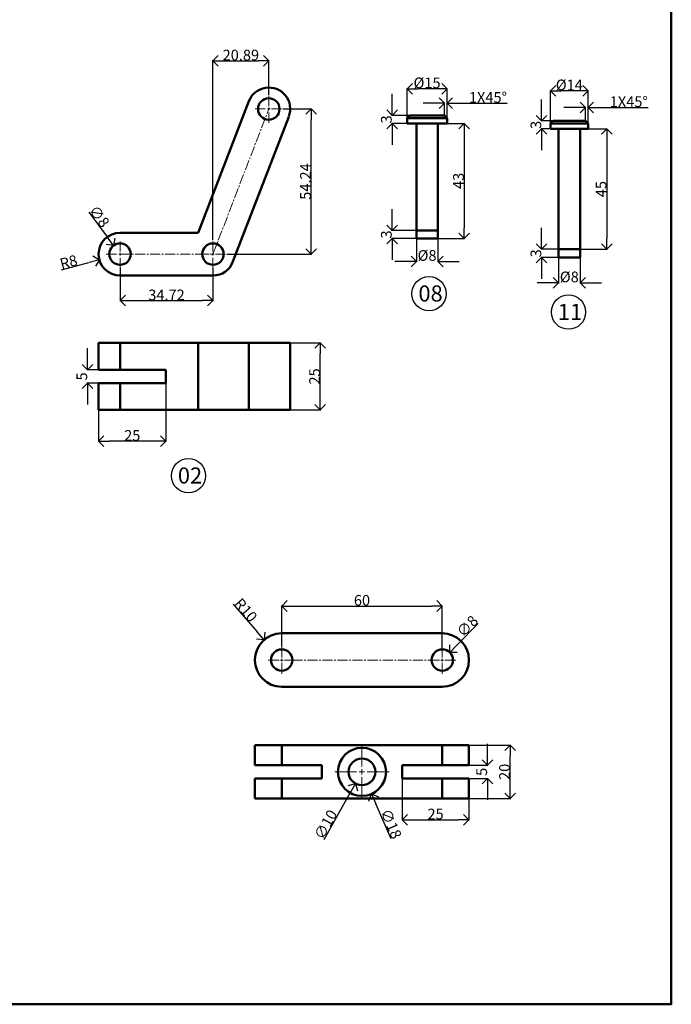
# Model space of a CAD drawing. Units: millimetres. Extents: x 45 to 546, y 51 to 638.
# Tile 2 of 4: x 303 to 546, y 51 to 419. Entities that reach past the tile are written whole.
import ezdxf

# ---------------------------------------------------------------- set-up
doc = ezdxf.new("R2010")
doc.units = ezdxf.units.MM
doc.header["$MEASUREMENT"] = 0
doc.linetypes.add('CENTER2', pattern=[1.125, 0.75, -0.125, 0.125, -0.125])
for name, color, linetype, lineweight in [('M-CNTR', 1, 'CENTER2', 18), ('M-DIMS', 2, 'Continuous', 25), ('M-OUTL', 7, 'Continuous', 50), ('M-TEXT', 7, 'Continuous', 25), ('M-TTLB', 7, 'Continuous', 50)]:
    doc.layers.add(name, color=color, linetype=linetype, lineweight=lineweight)
doc.styles.get("Standard").update_dxf_attribs({"font": 'arial.ttf'})
doc.dimstyles.get("Standard").update_dxf_attribs({"dimtxt": 4, "dimasz": 4, "dimexe": 0.18, "dimexo": 0.0625, "dimgap": 0.09, "dimtad": 1, "dimdec": 0, "dimzin": 0, "dimdsep": 46, "dimtxsty": 'Standard', "dimblk": 'OPEN90', "dimcen": 0.09, "dimclre": 251, "dimadec": 0, "dimazin": 0, "dimtfac": 1, "dimtdec": 0, "dimtofl": 0, "dimtmove": 0, "dimatfit": 3, "dimfxl": 1, "dimtolj": 1, "dimtzin": 0, "dimarcsym": 0})

# ---------------------------------------------------------------- blocks, each defined once
blk = doc.blocks.new('_Open90')
at = {"color": 0, "linetype": 'ByBlock', "lineweight": -2}
for p, q in [((0, 0), (-1, 0)), ((-0.5, 0.5), (0, 0)), ((0, 0), (-0.5, -0.5))]:
    blk.add_line(p, q, dxfattribs=at)
blk = doc.blocks.new('*D54')
at = {"layer": 'Defpoints', "color": 0, "transparency": 16777216}
for p in [(337.79, 334.56), (342.59, 328.16)]:
    blk.add_point(p, dxfattribs=at)
at = {"layer": 'M-DIMS', "color": 0, "lineweight": -2, "transparency": 16777216}
for p, q in [((328.48, 346.98), (335.39, 337.76)), ((340.1, 331.36), (340.28, 331.36)), ((340.19, 331.27), (340.19, 331.45))]:
    blk.add_line(p, q, dxfattribs=at)
at = {"layer": 'M-DIMS', "color": 0, "lineweight": -2, "transparency": 16777216, "xscale": 4, "yscale": 4, "zscale": 4, "rotation": 306.8480275512002}
blk.add_blockref('_Open90', (337.79, 334.56), dxfattribs=at)
at = {"layer": 'M-DIMS', "color": 0, "transparency": 16777216, "insert": (332.42, 345.46), "char_height": 4, "attachment_point": 5, "rotation": 306.848}
blk.add_mtext('\\A1;∅8', dxfattribs=at)
blk = doc.blocks.new('*D55')
at = {"layer": 'Defpoints', "color": 0, "transparency": 16777216}
for p in [(340.19, 331.36), (332.46, 329.29)]:
    blk.add_point(p, dxfattribs=at)
at = {"layer": 'M-DIMS', "color": 0, "lineweight": -2, "transparency": 16777216}
for p, q in [((340.1, 331.36), (340.28, 331.36)), ((340.19, 331.27), (340.19, 331.45)), ((318.32, 325.51), (328.59, 328.26))]:
    blk.add_line(p, q, dxfattribs=at)
at = {"layer": 'M-DIMS', "color": 0, "lineweight": -2, "transparency": 16777216, "xscale": 4, "yscale": 4, "zscale": 4, "rotation": 14.96151981940441}
blk.add_blockref('_Open90', (332.46, 329.29), dxfattribs=at)
at = {"layer": 'M-DIMS', "color": 0, "transparency": 16777216, "insert": (320.97, 328.43), "char_height": 4, "attachment_point": 5, "rotation": 14.9615}
blk.add_mtext('\\A1;R8', dxfattribs=at)
blk = doc.blocks.new('*U56')
at = {"layer": 'M-CNTR', "color": 0, "ltscale": 5, "transparency": 16777216}
for p, q in [((0, 1), (0, 5.12)), ((-5.12, 0), (-1, 0)), ((1, 0), (5.12, 0)), ((0, -5.12), (0, -1))]:
    blk.add_line(p, q, dxfattribs=at)
at = {"layer": 'M-CNTR', "color": 0, "linetype": 'Continuous', "ltscale": 5, "transparency": 16777216}
for p, q in [((-0.5, 0), (0.5, 0)), ((0, -0.5), (0, 0.5))]:
    blk.add_line(p, q, dxfattribs=at)
blk = doc.blocks.new('*U57')
at = {"layer": 'M-CNTR', "color": 0, "ltscale": 5, "transparency": 16777216}
for p, q in [((0, 1), (0, 5.12)), ((-5.12, 0), (-1, 0)), ((1, 0), (5.12, 0)), ((0, -5.12), (0, -1))]:
    blk.add_line(p, q, dxfattribs=at)
at = {"layer": 'M-CNTR', "color": 0, "linetype": 'Continuous', "ltscale": 5, "transparency": 16777216}
for p, q in [((-0.5, 0), (0.5, 0)), ((0, -0.5), (0, 0.5))]:
    blk.add_line(p, q, dxfattribs=at)
blk = doc.blocks.new('*U58')
at = {"layer": 'M-CNTR', "color": 0, "ltscale": 5, "transparency": 16777216}
for p, q in [((0, 1), (0, 5.12)), ((-5.12, 0), (-1, 0)), ((1, 0), (5.12, 0)), ((0, -5.12), (0, -1))]:
    blk.add_line(p, q, dxfattribs=at)
at = {"layer": 'M-CNTR', "color": 0, "linetype": 'Continuous', "ltscale": 5, "transparency": 16777216}
for p, q in [((-0.5, 0), (0.5, 0)), ((0, -0.5), (0, 0.5))]:
    blk.add_line(p, q, dxfattribs=at)
blk = doc.blocks.new('*D59')
at = {"layer": 'Defpoints', "color": 0, "transparency": 16777216}
for p in [(340.19, 326.24), (374.91, 326.24), (374.91, 313.98)]:
    blk.add_point(p, dxfattribs=at)
at = {"layer": 'M-DIMS', "color": 0, "lineweight": -2, "transparency": 16777216}
for p, q in [((340.19, 326.18), (340.19, 313.8)), ((374.91, 326.18), (374.91, 313.8)), ((344.19, 313.98), (370.91, 313.98))]:
    blk.add_line(p, q, dxfattribs=at)
at = {"layer": 'M-DIMS', "color": 0, "lineweight": -2, "transparency": 16777216, "xscale": 4, "yscale": 4, "zscale": 4, "rotation": 180}
blk.add_blockref('_Open90', (340.19, 313.98), dxfattribs=at)
at = {"layer": 'M-DIMS', "color": 0, "lineweight": -2, "transparency": 16777216, "xscale": 4, "yscale": 4, "zscale": 4}
blk.add_blockref('_Open90', (374.91, 313.98), dxfattribs=at)
at = {"layer": 'M-DIMS', "color": 0, "transparency": 16777216, "insert": (357.55, 316.11), "char_height": 4, "attachment_point": 5}
blk.add_mtext('\\A1;34.72', dxfattribs=at)
blk = doc.blocks.new('*D60')
at = {"layer": 'Defpoints', "color": 0, "transparency": 16777216}
for p in [(400.92, 385.6), (411.64, 385.6), (380.03, 331.36)]:
    blk.add_point(p, dxfattribs=at)
at = {"layer": 'M-DIMS', "color": 0, "lineweight": -2, "transparency": 16777216}
for p, q in [((400.98, 385.6), (411.82, 385.6)), ((411.64, 335.36), (411.64, 381.6)), ((380.09, 331.36), (411.82, 331.36))]:
    blk.add_line(p, q, dxfattribs=at)
at = {"layer": 'M-DIMS', "color": 0, "lineweight": -2, "transparency": 16777216, "xscale": 4, "yscale": 4, "zscale": 4}
for p, rotation in [((411.64, 385.6), 90), ((411.64, 331.36), 270)]:
    blk.add_blockref('_Open90', p, dxfattribs=dict(at, rotation=rotation))
at = {"layer": 'M-DIMS', "color": 0, "transparency": 16777216, "insert": (409.5, 358.48), "char_height": 4, "attachment_point": 5, "rotation": 90}
blk.add_mtext('\\A1;54.24', dxfattribs=at)
blk = doc.blocks.new('*D61')
at = {"layer": 'Defpoints', "color": 0, "transparency": 16777216}
for p in [(395.8, 403.6), (395.8, 390.72), (374.91, 336.48)]:
    blk.add_point(p, dxfattribs=at)
at = {"layer": 'M-DIMS', "color": 0, "lineweight": -2, "transparency": 16777216}
for p, q in [((374.91, 336.54), (374.91, 403.78)), ((378.91, 403.6), (391.8, 403.6)), ((395.8, 390.78), (395.8, 403.78))]:
    blk.add_line(p, q, dxfattribs=at)
at = {"layer": 'M-DIMS', "color": 0, "lineweight": -2, "transparency": 16777216, "xscale": 4, "yscale": 4, "zscale": 4, "rotation": 180}
blk.add_blockref('_Open90', (374.91, 403.6), dxfattribs=at)
at = {"layer": 'M-DIMS', "color": 0, "lineweight": -2, "transparency": 16777216, "xscale": 4, "yscale": 4, "zscale": 4}
blk.add_blockref('_Open90', (395.8, 403.6), dxfattribs=at)
at = {"layer": 'M-DIMS', "color": 0, "transparency": 16777216, "insert": (385.35, 405.73), "char_height": 4, "attachment_point": 5}
blk.add_mtext('\\A1;20.89', dxfattribs=at)
blk = doc.blocks.new('*D62')
at = {"layer": 'Defpoints', "color": 0, "transparency": 16777216}
for p in [(328.02, 288.16), (332.19, 288.16), (332.19, 283.16)]:
    blk.add_point(p, dxfattribs=at)
at = {"layer": 'M-DIMS', "color": 0, "lineweight": -2, "transparency": 16777216}
for p, q in [((328.02, 292.16), (328.02, 296.16)), ((332.13, 288.16), (327.84, 288.16)), ((332.13, 283.16), (327.84, 283.16)), ((328.02, 279.16), (328.02, 275.16))]:
    blk.add_line(p, q, dxfattribs=at)
at = {"layer": 'M-DIMS', "color": 0, "lineweight": -2, "transparency": 16777216, "xscale": 4, "yscale": 4, "zscale": 4}
for p, rotation in [((328.02, 288.16), 270), ((328.02, 283.16), 90)]:
    blk.add_blockref('_Open90', p, dxfattribs=dict(at, rotation=rotation))
at = {"layer": 'M-DIMS', "color": 0, "transparency": 16777216, "insert": (325.9, 285.66), "char_height": 4, "attachment_point": 5, "rotation": 90}
blk.add_mtext('\\A1;5', dxfattribs=at)
blk = doc.blocks.new('*D63')
at = {"layer": 'Defpoints', "color": 0, "transparency": 16777216}
for p in [(357.34, 283.16), (332.19, 273.16), (332.19, 261.47)]:
    blk.add_point(p, dxfattribs=at)
at = {"layer": 'M-DIMS', "color": 0, "lineweight": -2, "transparency": 16777216}
for p, q in [((357.34, 283.1), (357.34, 261.29)), ((332.19, 273.1), (332.19, 261.29)), ((353.34, 261.47), (336.19, 261.47))]:
    blk.add_line(p, q, dxfattribs=at)
at = {"layer": 'M-DIMS', "color": 0, "lineweight": -2, "transparency": 16777216, "xscale": 4, "yscale": 4, "zscale": 4, "rotation": 180}
blk.add_blockref('_Open90', (332.19, 261.47), dxfattribs=at)
at = {"layer": 'M-DIMS', "color": 0, "lineweight": -2, "transparency": 16777216, "xscale": 4, "yscale": 4, "zscale": 4}
blk.add_blockref('_Open90', (357.34, 261.47), dxfattribs=at)
at = {"layer": 'M-DIMS', "color": 0, "transparency": 16777216, "insert": (344.76, 263.6), "char_height": 4, "attachment_point": 5}
blk.add_mtext('\\A1;25', dxfattribs=at)
blk = doc.blocks.new('*D64')
at = {"layer": 'Defpoints', "color": 0, "transparency": 16777216}
for p in [(403.8, 298.16), (415.04, 298.16), (403.8, 273.16)]:
    blk.add_point(p, dxfattribs=at)
at = {"layer": 'M-DIMS', "color": 0, "lineweight": -2, "transparency": 16777216}
for p, q in [((403.86, 298.16), (415.22, 298.16)), ((415.04, 277.16), (415.04, 294.16)), ((403.86, 273.16), (415.22, 273.16))]:
    blk.add_line(p, q, dxfattribs=at)
at = {"layer": 'M-DIMS', "color": 0, "lineweight": -2, "transparency": 16777216, "xscale": 4, "yscale": 4, "zscale": 4}
for p, rotation in [((415.04, 298.16), 90), ((415.04, 273.16), 270)]:
    blk.add_blockref('_Open90', p, dxfattribs=dict(at, rotation=rotation))
at = {"layer": 'M-DIMS', "color": 0, "transparency": 16777216, "insert": (412.91, 285.66), "char_height": 4, "attachment_point": 5, "rotation": 90}
blk.add_mtext('\\A1;25', dxfattribs=at)
blk = doc.blocks.new('*D65')
at = {"layer": 'Defpoints', "color": 0, "transparency": 16777216}
for p in [(441.87, 383.22), (448.45, 383.22), (447.45, 380.22)]:
    blk.add_point(p, dxfattribs=at)
at = {"layer": 'M-DIMS', "color": 0, "lineweight": -2, "transparency": 16777216}
for p, q in [((441.87, 387.22), (441.87, 391.22)), ((448.39, 383.22), (441.69, 383.22)), ((447.39, 380.22), (441.69, 380.22)), ((441.87, 376.22), (441.87, 372.22))]:
    blk.add_line(p, q, dxfattribs=at)
at = {"layer": 'M-DIMS', "color": 0, "lineweight": -2, "transparency": 16777216, "xscale": 4, "yscale": 4, "zscale": 4}
for p, rotation in [((441.87, 383.22), 270), ((441.87, 380.22), 90)]:
    blk.add_blockref('_Open90', p, dxfattribs=dict(at, rotation=rotation))
at = {"layer": 'M-DIMS', "color": 0, "transparency": 16777216, "insert": (439.73, 381.72), "char_height": 4, "attachment_point": 5, "rotation": 90}
blk.add_mtext('\\A1;3', dxfattribs=at)
blk = doc.blocks.new('*D66')
at = {"layer": 'Defpoints', "color": 0, "transparency": 16777216}
for p in [(441.87, 340.22), (450.95, 340.22), (450.95, 337.22)]:
    blk.add_point(p, dxfattribs=at)
at = {"layer": 'M-DIMS', "color": 0, "lineweight": -2, "transparency": 16777216}
for p, q in [((441.87, 344.22), (441.87, 348.22)), ((450.89, 340.22), (441.69, 340.22)), ((450.89, 337.22), (441.69, 337.22)), ((441.87, 333.22), (441.87, 329.22))]:
    blk.add_line(p, q, dxfattribs=at)
at = {"layer": 'M-DIMS', "color": 0, "lineweight": -2, "transparency": 16777216, "xscale": 4, "yscale": 4, "zscale": 4}
for p, rotation in [((441.87, 340.22), 270), ((441.87, 337.22), 90)]:
    blk.add_blockref('_Open90', p, dxfattribs=dict(at, rotation=rotation))
at = {"layer": 'M-DIMS', "color": 0, "transparency": 16777216, "insert": (439.73, 338.72), "char_height": 4, "attachment_point": 5, "rotation": 90}
blk.add_mtext('\\A1;3', dxfattribs=at)
blk = doc.blocks.new('*D67')
at = {"layer": 'Defpoints', "color": 0, "transparency": 16777216}
for p in [(462.45, 380.22), (458.95, 337.22), (468.81, 337.22)]:
    blk.add_point(p, dxfattribs=at)
at = {"layer": 'M-DIMS', "color": 0, "lineweight": -2, "transparency": 16777216}
for p, q in [((462.52, 380.22), (468.99, 380.22)), ((468.81, 376.22), (468.81, 341.22)), ((459.02, 337.22), (468.99, 337.22))]:
    blk.add_line(p, q, dxfattribs=at)
at = {"layer": 'M-DIMS', "color": 0, "lineweight": -2, "transparency": 16777216, "xscale": 4, "yscale": 4, "zscale": 4}
for p, rotation in [((468.81, 380.22), 90), ((468.81, 337.22), 270)]:
    blk.add_blockref('_Open90', p, dxfattribs=dict(at, rotation=rotation))
at = {"layer": 'M-DIMS', "color": 0, "transparency": 16777216, "insert": (466.68, 358.72), "char_height": 4, "attachment_point": 5, "rotation": 90}
blk.add_mtext('\\A1;43', dxfattribs=at)
blk = doc.blocks.new('*D68')
at = {"layer": 'Defpoints', "color": 0, "transparency": 16777216}
for p in [(450.95, 337.22), (458.95, 337.22), (450.95, 328.62)]:
    blk.add_point(p, dxfattribs=at)
at = {"layer": 'M-DIMS', "color": 0, "lineweight": -2, "transparency": 16777216}
for p, q in [((450.95, 337.16), (450.95, 328.44)), ((458.95, 337.16), (458.95, 328.44)), ((446.95, 328.62), (442.95, 328.62)), ((462.95, 328.62), (466.95, 328.62))]:
    blk.add_line(p, q, dxfattribs=at)
at = {"layer": 'M-DIMS', "color": 0, "lineweight": -2, "transparency": 16777216, "xscale": 4, "yscale": 4, "zscale": 4}
blk.add_blockref('_Open90', (450.95, 328.62), dxfattribs=at)
at = {"layer": 'M-DIMS', "color": 0, "lineweight": -2, "transparency": 16777216, "xscale": 4, "yscale": 4, "zscale": 4, "rotation": 180}
blk.add_blockref('_Open90', (458.95, 328.62), dxfattribs=at)
at = {"layer": 'M-DIMS', "color": 0, "transparency": 16777216, "insert": (454.95, 330.86), "char_height": 4, "attachment_point": 5}
blk.add_mtext('\\A1;%%C8', dxfattribs=at)
blk = doc.blocks.new('*D69')
at = {"layer": 'Defpoints', "color": 0, "transparency": 16777216}
for p in [(447.45, 393.11), (447.45, 382.22), (462.45, 382.22)]:
    blk.add_point(p, dxfattribs=at)
at = {"layer": 'M-DIMS', "color": 0, "lineweight": -2, "transparency": 16777216}
for p, q in [((447.45, 382.28), (447.45, 393.29)), ((458.45, 393.11), (451.45, 393.11)), ((462.45, 382.28), (462.45, 393.29))]:
    blk.add_line(p, q, dxfattribs=at)
at = {"layer": 'M-DIMS', "color": 0, "lineweight": -2, "transparency": 16777216, "xscale": 4, "yscale": 4, "zscale": 4, "rotation": 180}
blk.add_blockref('_Open90', (447.45, 393.11), dxfattribs=at)
at = {"layer": 'M-DIMS', "color": 0, "lineweight": -2, "transparency": 16777216, "xscale": 4, "yscale": 4, "zscale": 4}
blk.add_blockref('_Open90', (462.45, 393.11), dxfattribs=at)
at = {"layer": 'M-DIMS', "color": 0, "transparency": 16777216, "insert": (454.95, 395.35), "char_height": 4, "attachment_point": 5}
blk.add_mtext('\\A1;%%C15', dxfattribs=at)
blk = doc.blocks.new('*D70')
at = {"layer": 'Defpoints', "color": 0, "transparency": 16777216}
for p in [(462.45, 387.79), (461.45, 383.22), (462.45, 382.22)]:
    blk.add_point(p, dxfattribs=at)
at = {"layer": 'M-DIMS', "color": 0, "lineweight": -2, "transparency": 16777216}
for p, q in [((457.45, 387.79), (453.45, 387.79)), ((461.45, 383.28), (461.45, 387.97)), ((462.45, 382.28), (462.45, 387.97)), ((466.45, 387.79), (484.94, 387.79))]:
    blk.add_line(p, q, dxfattribs=at)
at = {"layer": 'M-DIMS', "color": 0, "lineweight": -2, "transparency": 16777216, "xscale": 4, "yscale": 4, "zscale": 4}
blk.add_blockref('_Open90', (461.45, 387.79), dxfattribs=at)
at = {"layer": 'M-DIMS', "color": 0, "lineweight": -2, "transparency": 16777216, "xscale": 4, "yscale": 4, "zscale": 4, "rotation": 180}
blk.add_blockref('_Open90', (462.45, 387.79), dxfattribs=at)
at = {"layer": 'M-DIMS', "color": 0, "transparency": 16777216, "insert": (477.7, 389.92), "char_height": 4, "attachment_point": 5}
blk.add_mtext('\\A1;1X45%%D', dxfattribs=at)
blk = doc.blocks.new('*D71')
at = {"layer": 'Defpoints', "color": 0, "transparency": 16777216}
for p in [(497.77, 333.16), (504.11, 333.16), (504.11, 330.16)]:
    blk.add_point(p, dxfattribs=at)
at = {"layer": 'M-DIMS', "color": 0, "lineweight": -2, "transparency": 16777216}
for p, q in [((497.77, 337.16), (497.77, 341.16)), ((504.05, 333.16), (497.59, 333.16)), ((504.05, 330.16), (497.59, 330.16)), ((497.77, 326.16), (497.77, 322.16))]:
    blk.add_line(p, q, dxfattribs=at)
at = {"layer": 'M-DIMS', "color": 0, "lineweight": -2, "transparency": 16777216, "xscale": 4, "yscale": 4, "zscale": 4}
for p, rotation in [((497.77, 333.16), 270), ((497.77, 330.16), 90)]:
    blk.add_blockref('_Open90', p, dxfattribs=dict(at, rotation=rotation))
at = {"layer": 'M-DIMS', "color": 0, "transparency": 16777216, "insert": (495.63, 331.66), "char_height": 4, "attachment_point": 5, "rotation": 90}
blk.add_mtext('\\A1;3', dxfattribs=at)
blk = doc.blocks.new('*D72')
at = {"layer": 'Defpoints', "color": 0, "transparency": 16777216}
for p in [(497.77, 381.16), (502.11, 381.16), (501.11, 378.16)]:
    blk.add_point(p, dxfattribs=at)
at = {"layer": 'M-DIMS', "color": 0, "lineweight": -2, "transparency": 16777216}
for p, q in [((497.77, 385.16), (497.77, 389.16)), ((502.05, 381.16), (497.59, 381.16)), ((501.05, 378.16), (497.59, 378.16)), ((497.77, 374.16), (497.77, 370.16))]:
    blk.add_line(p, q, dxfattribs=at)
at = {"layer": 'M-DIMS', "color": 0, "lineweight": -2, "transparency": 16777216, "xscale": 4, "yscale": 4, "zscale": 4}
for p, rotation in [((497.77, 381.16), 270), ((497.77, 378.16), 90)]:
    blk.add_blockref('_Open90', p, dxfattribs=dict(at, rotation=rotation))
at = {"layer": 'M-DIMS', "color": 0, "transparency": 16777216, "insert": (495.63, 379.66), "char_height": 4, "attachment_point": 5, "rotation": 90}
blk.add_mtext('\\A1;3', dxfattribs=at)
blk = doc.blocks.new('*D73')
at = {"layer": 'Defpoints', "color": 0, "transparency": 16777216}
for p in [(501.11, 392.34), (501.11, 380.16), (515.11, 380.16)]:
    blk.add_point(p, dxfattribs=at)
at = {"layer": 'M-DIMS', "color": 0, "lineweight": -2, "transparency": 16777216}
for p, q in [((501.11, 380.22), (501.11, 392.52)), ((511.11, 392.34), (505.11, 392.34)), ((515.11, 380.22), (515.11, 392.52))]:
    blk.add_line(p, q, dxfattribs=at)
at = {"layer": 'M-DIMS', "color": 0, "lineweight": -2, "transparency": 16777216, "xscale": 4, "yscale": 4, "zscale": 4, "rotation": 180}
blk.add_blockref('_Open90', (501.11, 392.34), dxfattribs=at)
at = {"layer": 'M-DIMS', "color": 0, "lineweight": -2, "transparency": 16777216, "xscale": 4, "yscale": 4, "zscale": 4}
blk.add_blockref('_Open90', (515.11, 392.34), dxfattribs=at)
at = {"layer": 'M-DIMS', "color": 0, "transparency": 16777216, "insert": (508.11, 394.58), "char_height": 4, "attachment_point": 5}
blk.add_mtext('\\A1;%%C14', dxfattribs=at)
blk = doc.blocks.new('*D74')
at = {"layer": 'Defpoints', "color": 0, "transparency": 16777216}
for p in [(515.11, 386.18), (514.11, 381.16), (515.11, 380.16)]:
    blk.add_point(p, dxfattribs=at)
at = {"layer": 'M-DIMS', "color": 0, "lineweight": -2, "transparency": 16777216}
for p, q in [((514.11, 381.22), (514.11, 386.36)), ((515.11, 380.22), (515.11, 386.36)), ((510.11, 386.18), (506.11, 386.18)), ((519.11, 386.18), (537.6, 386.18))]:
    blk.add_line(p, q, dxfattribs=at)
at = {"layer": 'M-DIMS', "color": 0, "lineweight": -2, "transparency": 16777216, "xscale": 4, "yscale": 4, "zscale": 4}
blk.add_blockref('_Open90', (514.11, 386.18), dxfattribs=at)
at = {"layer": 'M-DIMS', "color": 0, "lineweight": -2, "transparency": 16777216, "xscale": 4, "yscale": 4, "zscale": 4, "rotation": 180}
blk.add_blockref('_Open90', (515.11, 386.18), dxfattribs=at)
at = {"layer": 'M-DIMS', "color": 0, "transparency": 16777216, "insert": (530.35, 388.31), "char_height": 4, "attachment_point": 5}
blk.add_mtext('\\A1;1X45%%D', dxfattribs=at)
blk = doc.blocks.new('*D75')
at = {"layer": 'Defpoints', "color": 0, "transparency": 16777216}
for p in [(515.11, 378.16), (512.11, 333.16), (522.13, 333.16)]:
    blk.add_point(p, dxfattribs=at)
at = {"layer": 'M-DIMS', "color": 0, "lineweight": -2, "transparency": 16777216}
for p, q in [((515.17, 378.16), (522.31, 378.16)), ((522.13, 374.16), (522.13, 337.16)), ((512.17, 333.16), (522.31, 333.16))]:
    blk.add_line(p, q, dxfattribs=at)
at = {"layer": 'M-DIMS', "color": 0, "lineweight": -2, "transparency": 16777216, "xscale": 4, "yscale": 4, "zscale": 4}
for p, rotation in [((522.13, 378.16), 90), ((522.13, 333.16), 270)]:
    blk.add_blockref('_Open90', p, dxfattribs=dict(at, rotation=rotation))
at = {"layer": 'M-DIMS', "color": 0, "transparency": 16777216, "insert": (520, 355.66), "char_height": 4, "attachment_point": 5, "rotation": 90}
blk.add_mtext('\\A1;45', dxfattribs=at)
blk = doc.blocks.new('*D76')
at = {"layer": 'Defpoints', "color": 0, "transparency": 16777216}
for p in [(504.11, 330.16), (512.11, 330.16), (504.11, 320.61)]:
    blk.add_point(p, dxfattribs=at)
at = {"layer": 'M-DIMS', "color": 0, "lineweight": -2, "transparency": 16777216}
for p, q in [((504.11, 330.09), (504.11, 320.43)), ((512.11, 330.09), (512.11, 320.43)), ((500.11, 320.61), (496.11, 320.61)), ((516.11, 320.61), (520.11, 320.61))]:
    blk.add_line(p, q, dxfattribs=at)
at = {"layer": 'M-DIMS', "color": 0, "lineweight": -2, "transparency": 16777216, "xscale": 4, "yscale": 4, "zscale": 4}
blk.add_blockref('_Open90', (504.11, 320.61), dxfattribs=at)
at = {"layer": 'M-DIMS', "color": 0, "lineweight": -2, "transparency": 16777216, "xscale": 4, "yscale": 4, "zscale": 4, "rotation": 180}
blk.add_blockref('_Open90', (512.11, 320.61), dxfattribs=at)
at = {"layer": 'M-DIMS', "color": 0, "transparency": 16777216, "insert": (508.11, 322.85), "char_height": 4, "attachment_point": 5}
blk.add_mtext('\\A1;%%C8', dxfattribs=at)
blk = doc.blocks.new('*U101')
at = {"layer": 'M-CNTR', "color": 0, "transparency": 16777216}
for p, q in [((0, 1), (0, 5.12)), ((-5.12, 0), (-1, 0)), ((1, 0), (5.12, 0)), ((0, -5.12), (0, -1))]:
    blk.add_line(p, q, dxfattribs=at)
at = {"layer": 'M-CNTR', "color": 0, "linetype": 'Continuous', "transparency": 16777216}
for p, q in [((-0.5, 0), (0.5, 0)), ((0, -0.5), (0, 0.5))]:
    blk.add_line(p, q, dxfattribs=at)
blk = doc.blocks.new('*U102')
at = {"layer": 'M-CNTR', "color": 0, "transparency": 16777216}
for p, q in [((0, 1), (0, 5.12)), ((-5.12, 0), (-1, 0)), ((1, 0), (5.12, 0)), ((0, -5.12), (0, -1))]:
    blk.add_line(p, q, dxfattribs=at)
at = {"layer": 'M-CNTR', "color": 0, "linetype": 'Continuous', "transparency": 16777216}
for p, q in [((-0.5, 0), (0.5, 0)), ((0, -0.5), (0, 0.5))]:
    blk.add_line(p, q, dxfattribs=at)
blk = doc.blocks.new('*U103')
at = {"layer": 'M-CNTR', "color": 0, "transparency": 16777216}
for p, q in [((0, 2), (0, 10.12)), ((-10.12, 0), (-2, 0)), ((2, 0), (10.12, 0)), ((0, -10.12), (0, -2))]:
    blk.add_line(p, q, dxfattribs=at)
at = {"layer": 'M-CNTR', "color": 0, "linetype": 'Continuous', "transparency": 16777216}
for p, q in [((-1, 0), (1, 0)), ((0, -1), (0, 1))]:
    blk.add_line(p, q, dxfattribs=at)
blk = doc.blocks.new('*D104')
at = {"layer": 'Defpoints', "color": 0, "transparency": 16777216}
for p in [(460.62, 199.88), (400.62, 184.81), (460.62, 183.69)]:
    blk.add_point(p, dxfattribs=at)
at = {"layer": 'M-DIMS', "color": 0, "lineweight": -2, "transparency": 16777216}
for p, q in [((400.62, 184.87), (400.62, 200.06)), ((404.62, 199.88), (456.62, 199.88)), ((460.62, 183.75), (460.62, 200.06))]:
    blk.add_line(p, q, dxfattribs=at)
at = {"layer": 'M-DIMS', "color": 0, "lineweight": -2, "transparency": 16777216, "xscale": 4, "yscale": 4, "zscale": 4, "rotation": 180}
blk.add_blockref('_Open90', (400.62, 199.88), dxfattribs=at)
at = {"layer": 'M-DIMS', "color": 0, "lineweight": -2, "transparency": 16777216, "xscale": 4, "yscale": 4, "zscale": 4}
blk.add_blockref('_Open90', (460.62, 199.88), dxfattribs=at)
at = {"layer": 'M-DIMS', "color": 0, "transparency": 16777216, "insert": (430.62, 202.01), "char_height": 4, "attachment_point": 5}
blk.add_mtext('\\A1;60', dxfattribs=at)
blk = doc.blocks.new('*D105')
at = {"layer": 'Defpoints', "color": 0, "transparency": 16777216}
for p in [(394.06, 187.24), (400.62, 179.69)]:
    blk.add_point(p, dxfattribs=at)
at = {"layer": 'M-DIMS', "color": 0, "lineweight": -2, "transparency": 16777216}
for p, q in [((382.42, 200.61), (391.43, 190.26)), ((400.53, 179.69), (400.71, 179.69)), ((400.62, 179.6), (400.62, 179.78))]:
    blk.add_line(p, q, dxfattribs=at)
at = {"layer": 'M-DIMS', "color": 0, "lineweight": -2, "transparency": 16777216, "xscale": 4, "yscale": 4, "zscale": 4, "rotation": 311.0078137432373}
blk.add_blockref('_Open90', (394.06, 187.24), dxfattribs=at)
at = {"layer": 'M-DIMS', "color": 0, "transparency": 16777216, "insert": (387.22, 198.34), "char_height": 4, "attachment_point": 5, "rotation": 311.0078}
blk.add_mtext('\\A1;R10', dxfattribs=at)
blk = doc.blocks.new('*D106')
at = {"layer": 'Defpoints', "color": 0, "transparency": 16777216}
for p in [(463.43, 182.53), (457.8, 176.85)]:
    blk.add_point(p, dxfattribs=at)
at = {"layer": 'M-DIMS', "color": 0, "lineweight": -2, "transparency": 16777216}
for p, q in [((474.1, 193.31), (466.24, 185.38)), ((460.53, 179.69), (460.71, 179.69)), ((460.62, 179.6), (460.62, 179.78))]:
    blk.add_line(p, q, dxfattribs=at)
at = {"layer": 'M-DIMS', "color": 0, "lineweight": -2, "transparency": 16777216, "xscale": 4, "yscale": 4, "zscale": 4, "rotation": 225.2909511753125}
blk.add_blockref('_Open90', (463.43, 182.53), dxfattribs=at)
at = {"layer": 'M-DIMS', "color": 0, "transparency": 16777216, "insert": (469.98, 192.34), "char_height": 4, "attachment_point": 5, "rotation": 45.291}
blk.add_mtext('\\A1;∅8', dxfattribs=at)
blk = doc.blocks.new('*D107')
at = {"layer": 'Defpoints', "color": 0, "transparency": 16777216}
for p in [(427.03, 146.16), (434.21, 129.65)]:
    blk.add_point(p, dxfattribs=at)
at = {"layer": 'M-DIMS', "color": 0, "lineweight": -2, "transparency": 16777216}
for p, q in [((430.53, 137.91), (430.71, 137.91)), ((430.62, 137.82), (430.62, 138)), ((441.49, 112.9), (435.8, 125.98))]:
    blk.add_line(p, q, dxfattribs=at)
at = {"layer": 'M-DIMS', "color": 0, "lineweight": -2, "transparency": 16777216, "xscale": 4, "yscale": 4, "zscale": 4, "rotation": 113.5058917432133}
blk.add_blockref('_Open90', (434.21, 129.65), dxfattribs=at)
at = {"layer": 'M-DIMS', "color": 0, "transparency": 16777216, "insert": (441.5, 118.5), "char_height": 4, "attachment_point": 5, "rotation": 293.5059}
blk.add_mtext('\\A1;∅18', dxfattribs=at)
blk = doc.blocks.new('*D108')
at = {"layer": 'Defpoints', "color": 0, "transparency": 16777216}
for p in [(433.06, 142.27), (428.18, 133.54)]:
    blk.add_point(p, dxfattribs=at)
at = {"layer": 'M-DIMS', "color": 0, "lineweight": -2, "transparency": 16777216}
for p, q in [((430.53, 137.91), (430.71, 137.91)), ((430.62, 137.82), (430.62, 138)), ((416.5, 112.65), (426.22, 130.05))]:
    blk.add_line(p, q, dxfattribs=at)
at = {"layer": 'M-DIMS', "color": 0, "lineweight": -2, "transparency": 16777216, "xscale": 4, "yscale": 4, "zscale": 4, "rotation": 60.78777855053363}
blk.add_blockref('_Open90', (428.18, 133.54), dxfattribs=at)
at = {"layer": 'M-DIMS', "color": 0, "transparency": 16777216, "insert": (417.04, 118.22), "char_height": 4, "attachment_point": 5, "rotation": 60.7878}
blk.add_mtext('\\A1;∅10', dxfattribs=at)
blk = doc.blocks.new('*D109')
at = {"layer": 'Defpoints', "color": 0, "transparency": 16777216}
for p in [(445.62, 135.41), (470.62, 127.91), (470.62, 120.02)]:
    blk.add_point(p, dxfattribs=at)
at = {"layer": 'M-DIMS', "color": 0, "lineweight": -2, "transparency": 16777216}
for p, q in [((445.62, 135.34), (445.62, 119.84)), ((470.62, 127.84), (470.62, 119.84)), ((449.62, 120.02), (466.62, 120.02))]:
    blk.add_line(p, q, dxfattribs=at)
at = {"layer": 'M-DIMS', "color": 0, "lineweight": -2, "transparency": 16777216, "xscale": 4, "yscale": 4, "zscale": 4, "rotation": 180}
blk.add_blockref('_Open90', (445.62, 120.02), dxfattribs=at)
at = {"layer": 'M-DIMS', "color": 0, "lineweight": -2, "transparency": 16777216, "xscale": 4, "yscale": 4, "zscale": 4}
blk.add_blockref('_Open90', (470.62, 120.02), dxfattribs=at)
at = {"layer": 'M-DIMS', "color": 0, "transparency": 16777216, "insert": (458.12, 122.16), "char_height": 4, "attachment_point": 5}
blk.add_mtext('\\A1;25', dxfattribs=at)
blk = doc.blocks.new('*D110')
at = {"layer": 'Defpoints', "color": 0, "transparency": 16777216}
for p in [(470.62, 140.41), (477.49, 140.41), (470.62, 135.41)]:
    blk.add_point(p, dxfattribs=at)
at = {"layer": 'M-DIMS', "color": 0, "lineweight": -2, "transparency": 16777216}
for p, q in [((477.49, 144.41), (477.49, 148.41)), ((470.68, 140.41), (477.67, 140.41)), ((470.68, 135.41), (477.67, 135.41)), ((477.49, 131.41), (477.49, 127.41))]:
    blk.add_line(p, q, dxfattribs=at)
at = {"layer": 'M-DIMS', "color": 0, "lineweight": -2, "transparency": 16777216, "xscale": 4, "yscale": 4, "zscale": 4}
for p, rotation in [((477.49, 140.41), 270), ((477.49, 135.41), 90)]:
    blk.add_blockref('_Open90', p, dxfattribs=dict(at, rotation=rotation))
at = {"layer": 'M-DIMS', "color": 0, "transparency": 16777216, "insert": (475.37, 137.91), "char_height": 4, "attachment_point": 5, "rotation": 90}
blk.add_mtext('\\A1;5', dxfattribs=at)
blk = doc.blocks.new('*D111')
at = {"layer": 'Defpoints', "color": 0, "transparency": 16777216}
for p in [(470.62, 147.91), (486.03, 147.91), (470.62, 127.91)]:
    blk.add_point(p, dxfattribs=at)
at = {"layer": 'M-DIMS', "color": 0, "lineweight": -2, "transparency": 16777216}
for p, q in [((470.68, 147.91), (486.21, 147.91)), ((486.03, 131.91), (486.03, 143.91)), ((470.68, 127.91), (486.21, 127.91))]:
    blk.add_line(p, q, dxfattribs=at)
at = {"layer": 'M-DIMS', "color": 0, "lineweight": -2, "transparency": 16777216, "xscale": 4, "yscale": 4, "zscale": 4}
for p, rotation in [((486.03, 147.91), 90), ((486.03, 127.91), 270)]:
    blk.add_blockref('_Open90', p, dxfattribs=dict(at, rotation=rotation))
at = {"layer": 'M-DIMS', "color": 0, "transparency": 16777216, "insert": (483.9, 137.91), "char_height": 4, "attachment_point": 5, "rotation": 90}
blk.add_mtext('\\A1;20', dxfattribs=at)

msp = doc.modelspace()

# ---------------------------------------------------------------- linework, layer by layer
at = {"layer": 'M-CNTR', "ltscale": 5}
for p, q in [((374.908, 331.358), (395.798, 385.598)), ((340.188, 331.358), (374.908, 331.358)), ((404.617, 179.69), (456.617, 179.69))]:
    msp.add_line(p, q, dxfattribs=at)
at = {"layer": 'M-OUTL'}
for p, q in [((388.332, 388.473), (369.416, 339.358)), ((403.263, 382.722), (382.398, 328.548)), ((447.453, 382.22), (448.453, 383.22)), ((448.453, 383.22), (461.453, 383.22)), ((461.453, 383.22), (462.453, 382.22)), ((447.453, 382.22), (447.453, 380.22)), ((447.453, 382.22), (462.453, 382.22)), ((447.453, 380.22), (462.453, 380.22)), ((450.953, 380.22), (450.953, 337.22)), ((458.953, 380.22), (458.953, 337.22)), ((462.453, 380.22), (462.453, 382.22)), ((501.11, 380.157), (502.11, 381.157)), ((501.11, 380.157), (501.11, 378.157)), ((501.11, 380.157), (515.11, 380.157)), ((502.11, 381.157), (514.11, 381.157)), ((514.11, 381.157), (515.11, 380.157)), ((515.11, 378.157), (515.11, 380.157)), ((501.11, 378.157), (515.11, 378.157)), ((504.11, 378.157), (504.11, 330.157)), ((512.11, 378.157), (512.11, 330.157)), ((369.416, 339.358), (340.188, 339.358)), ((450.953, 340.22), (458.953, 340.22)), ((450.953, 337.22), (458.953, 337.22)), ((504.11, 333.157), (512.11, 333.157)), ((504.11, 330.157), (512.11, 330.157)), ((340.188, 323.358), (374.908, 323.358)), ((332.188, 298.16), (403.798, 298.16)), ((332.188, 288.16), (332.188, 298.16)), ((340.188, 288.16), (340.188, 298.16)), ((369.416, 273.16), (369.416, 298.16)), ((388.332, 273.16), (388.332, 298.16)), ((403.798, 273.16), (403.798, 298.16)), ((357.338, 288.16), (332.188, 288.16)), ((357.338, 283.16), (357.338, 288.16)), ((332.188, 273.16), (332.188, 283.16)), ((357.338, 283.16), (332.188, 283.16)), ((357.338, 283.16), (332.188, 283.16)), ((340.188, 273.16), (340.188, 283.16)), ((332.188, 273.16), (403.798, 273.16)), ((400.617, 189.69), (460.617, 189.69)), ((400.617, 169.69), (460.617, 169.69)), ((390.617, 147.906), (470.617, 147.906)), ((390.617, 140.406), (390.617, 147.906)), ((400.617, 147.906), (400.617, 140.406)), ((460.617, 140.406), (460.617, 147.906)), ((470.617, 140.406), (470.617, 147.906)), ((390.617, 140.406), (415.617, 140.406)), ((415.617, 135.406), (415.617, 140.406)), ((445.617, 135.406), (445.617, 140.406)), ((445.617, 140.406), (470.617, 140.406)), ((390.617, 127.906), (390.617, 135.406)), ((390.617, 135.406), (415.617, 135.406)), ((400.617, 135.406), (400.617, 127.906)), ((445.617, 135.406), (470.617, 135.406)), ((460.617, 135.406), (460.617, 127.906)), ((470.617, 127.906), (470.617, 135.406)), ((390.617, 127.906), (470.617, 127.906))]:
    msp.add_line(p, q, dxfattribs=at)
for centre, radius in [((395.798, 385.598), 4), ((340.188, 331.358), 4), ((374.908, 331.358), 4), ((400.617, 179.69), 4), ((460.617, 179.69), 4), ((430.617, 137.906), 9), ((430.617, 137.906), 5)]:
    msp.add_circle(centre, radius, dxfattribs=at)
for centre, radius, start, end in [((395.798, 385.598), 8, 338.936, 158.936), ((340.188, 331.358), 8, 90, 270), ((374.908, 331.358), 8, 270, 339.43868), ((400.617, 179.69), 10, 90, 270), ((460.617, 179.69), 10, 270, 90)]:
    msp.add_arc(centre, radius, start, end, dxfattribs=at)
at = {"layer": 'M-TEXT'}
for centre in [(455.695, 316.565), (507.803, 309.691), (365.774, 248.552)]:
    msp.add_circle(centre, 6.408, dxfattribs=at)
at = {"layer": 'M-TTLB'}
msp.add_lwpolyline([(45.357, 637.893), (546.237, 637.893), (546.237, 51.054), (45.357, 51.054)], close=True, dxfattribs=at)

# ---------------------------------------------------------------- block references
at = {"layer": 'M-CNTR', "ltscale": 5}
for name, p in [('*U56', (395.798, 385.598)), ('*U57', (340.188, 331.358)), ('*U58', (374.908, 331.358))]:
    msp.add_blockref(name, p, dxfattribs=at)
at = {"layer": 'M-CNTR'}
for name, p in [('*U102', (400.617, 179.69)), ('*U101', (460.617, 179.69)), ('*U103', (430.617, 137.906))]:
    msp.add_blockref(name, p, dxfattribs=at)

# ---------------------------------------------------------------- texts
at = {"layer": 'M-TEXT', "char_height": 6, "attachment_point": 1}
for s, insert in [('08', (451.715, 319.661)), ('11', (503.824, 312.787)), ('02', (361.795, 251.648))]:
    msp.add_mtext_dynamic_manual_height_columns(s, width=105.49417, gutter_width=1, heights=[0], dxfattribs=dict(at, insert=insert))

# ---------------------------------------------------------------- dimensions: what is measured, and where the dimension line sits
at = {"layer": 'M-DIMS'}
for base, p1, p2, override, picture, middle in [((395.798, 403.6), (374.908, 336.478), (395.798, 390.718), {"dimdec": 2, "dimclrd": 0, "dimclre": 0, "dimclrt": 0}, '*D61', (385.353, 405.733)), ((374.908, 313.978), (340.188, 326.238), (374.908, 326.238), {"dimdec": 2, "dimclrd": 0, "dimclre": 0, "dimclrt": 0}, '*D59', (357.548, 316.111)), ((332.188, 261.469), (357.338, 283.16), (332.188, 273.16), {"dimclrd": 0, "dimclre": 0, "dimclrt": 0}, '*D63', (344.763, 263.601)), ((460.617, 199.876), (400.617, 184.81), (460.617, 183.69), {"dimclrd": 0, "dimclre": 0, "dimclrt": 0}, '*D104', (430.617, 202.008)), ((470.617, 120.024), (445.617, 135.406), (470.617, 127.906), {"dimclrd": 0, "dimclre": 0, "dimclrt": 0}, '*D109', (458.117, 122.157))]:
    dim = msp.add_linear_dim(base=base, p1=p1, p2=p2, dimstyle='Standard', override=override, dxfattribs=at)
    dim.commit()
    dim.dimension.update_dxf_attribs({"geometry": picture, "text_midpoint": middle})
for base, p1, p2, text, picture, middle in [((447.453, 393.108), (462.453, 382.22), (447.453, 382.22), '%%C<>', '*D69', (454.953, 395.353)), ((501.11, 392.339), (515.11, 380.157), (501.11, 380.157), '%%C<>', '*D73', (508.11, 394.584)), ((462.453, 387.785), (461.453, 383.22), (462.453, 382.22), '<>X45%%D', '*D70', (477.696, 389.918)), ((515.11, 386.179), (514.11, 381.157), (515.11, 380.157), '<>X45%%D', '*D74', (530.353, 388.311)), ((450.953, 328.618), (458.953, 337.22), (450.953, 337.22), '%%C<>', '*D68', (454.953, 330.862)), ((504.11, 320.605), (512.11, 330.157), (504.11, 330.157), '%%C<>', '*D76', (508.11, 322.849))]:
    dim = msp.add_linear_dim(base=base, p1=p1, p2=p2, text=text, dimstyle='Standard', override={"dimclrd": 0, "dimclre": 0, "dimclrt": 0}, dxfattribs=at)
    dim.commit()
    dim.dimension.update_dxf_attribs({"geometry": picture, "text_midpoint": middle})
for base, p1, p2, override, picture, middle in [((441.866, 383.22), (447.453, 380.22), (448.453, 383.22), {"dimclrd": 0, "dimclre": 0, "dimclrt": 0}, '*D65', (439.733, 381.72)), ((497.769, 381.157), (501.11, 378.157), (502.11, 381.157), {"dimclrd": 0, "dimclre": 0, "dimclrt": 0}, '*D72', (495.635, 379.657)), ((411.637, 385.598), (380.028, 331.358), (400.918, 385.598), {"dimdec": 2, "dimclrd": 0, "dimclre": 0, "dimclrt": 0}, '*D60', (409.504, 358.478)), ((468.811, 337.22), (462.453, 380.22), (458.953, 337.22), {"dimclrd": 0, "dimclre": 0, "dimclrt": 0}, '*D67', (466.677, 358.72)), ((522.126, 333.157), (515.11, 378.157), (512.11, 333.157), {"dimclrd": 0, "dimclre": 0, "dimclrt": 0}, '*D75', (520.002, 355.657)), ((441.866, 340.22), (450.953, 337.22), (450.953, 340.22), {"dimclrd": 0, "dimclre": 0, "dimclrt": 0}, '*D66', (439.733, 338.72)), ((497.769, 333.157), (504.11, 330.157), (504.11, 333.157), {"dimclrd": 0, "dimclre": 0, "dimclrt": 0}, '*D71', (495.635, 331.657)), ((415.041, 298.16), (403.798, 273.16), (403.798, 298.16), {"dimclrd": 0, "dimclre": 0, "dimclrt": 0}, '*D64', (412.909, 285.66)), ((328.024, 288.16), (332.188, 283.16), (332.188, 288.16), {"dimclrd": 0, "dimclre": 0, "dimclrt": 0}, '*D62', (325.9, 285.66)), ((477.494, 140.406), (470.617, 135.406), (470.617, 140.406), {"dimclrd": 0, "dimclre": 0, "dimclrt": 0}, '*D110', (475.37, 137.906)), ((486.034, 147.906), (470.617, 127.906), (470.617, 147.906), {"dimclrd": 0, "dimclre": 0, "dimclrt": 0}, '*D111', (483.902, 137.906))]:
    dim = msp.add_linear_dim(base=base, p1=p1, p2=p2, angle=90, dimstyle='Standard', override=override, dxfattribs=at)
    dim.commit()
    dim.dimension.update_dxf_attribs({"geometry": picture, "text_midpoint": middle})
for p1, p2, picture, middle in [((342.587, 328.157), (337.789, 334.559), '*D54', (330.625, 344.118)), ((433.057, 142.27), (428.176, 133.542), '*D108', (418.997, 117.125))]:
    dim = msp.add_diameter_dim_2p(p1=p1, p2=p2, dimstyle='Standard', override={"dimclrd": 0, "dimclre": 0, "dimclrt": 0}, dxfattribs=at)
    dim.commit()
    dim.dimension.update_dxf_attribs({"geometry": picture, "text_midpoint": middle, "dimtype": 163})
for center, mpoint, picture, middle in [((340.188, 331.358), (332.459, 329.292), '*D55', (320.973, 328.43)), ((400.617, 179.69), (394.055, 187.237), '*D105', (387.224, 198.342))]:
    dim = msp.add_radius_dim(center=center, mpoint=mpoint, dimstyle='Standard', override={"dimclrd": 0, "dimclre": 0, "dimclrt": 0}, dxfattribs=at)
    dim.commit()
    dim.dimension.update_dxf_attribs({"geometry": picture, "text_midpoint": middle})
for p1, p2, picture, middle in [((457.803, 176.848), (463.431, 182.533), '*D106', (469.983, 192.343)), ((427.027, 146.159), (434.206, 129.653), '*D107', (441.503, 118.503))]:
    dim = msp.add_diameter_dim_2p(p1=p1, p2=p2, dimstyle='Standard', override={"dimclrd": 0, "dimclre": 0, "dimclrt": 0}, dxfattribs=at)
    dim.commit()
    dim.dimension.update_dxf_attribs({"geometry": picture, "text_midpoint": middle})

doc.saveas('drawing.dxf')
